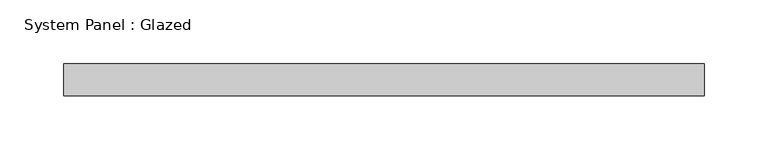
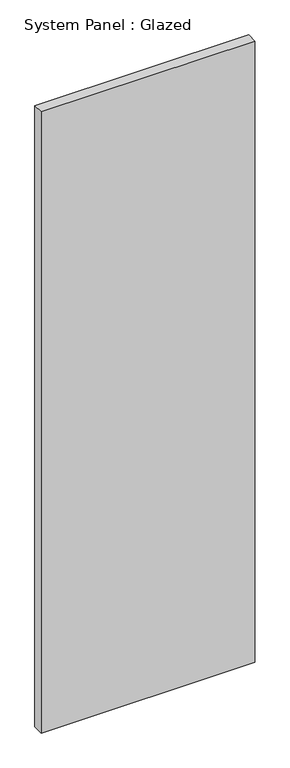
"""IFC4 building model written with IfcOpenShell, lengths in millimetres: plate geometry, System Panel : Glazed."""

from ifc_helpers import new_model, si_unit, origin, origin_with_axes, place, context, project, spatial, polyline, outline, extrude, source, transform, mapped, element, save


def system_panel_glazed_66bb8edf(model_context):
    return source(origin(), model_context, "Body", "SweptSolid", [
        extrude(outline(polyline([(251.8833333, 19.05), (-251.8833333, 19.05), (-251.8833333, 44.45), (251.8833333, 44.45), (251.8833333, 19.05)])), origin_with_axes(), (0.0, 0.0, 1.0), 1548.2875727),
    ])


if __name__ == "__main__":
    model = new_model("IFC4")
    model_context = context("Model", 3, world=origin())
    ifc_project = project(units=[si_unit("LENGTHUNIT", "METRE", prefix="MILLI")], contexts=[model_context])
    site = spatial("IfcSite", under=ifc_project)
    building = spatial("IfcBuilding", under=site)
    placement = place(None, origin())
    system_panel_glazed_shape = system_panel_glazed_66bb8edf(model_context)
    element("IfcPlate", 1, ObjectType="System Panel : Glazed", at=placement, inside=building, context=model_context, shape_type="MappedRepresentation", body=[
        mapped(system_panel_glazed_shape, transform((0.0, 0.0, 0.0), x_axis=(1.0, 0.0, 0.0), y_axis=(0.0, 1.0, 0.0), z_axis=(0.0, 0.0, 1.0))),
    ])
    save(model, "model.ifc")

# Revit data of these elements
# Type "System Panel : Glazed"
#   Construction Type Id = "GSP4R"
#   Analytic Construction = "1/8 in Pilkington single glazing"
#   Visual Light Transmittance = 0.9
#   Solar Heat Gain Coefficient = 0.86
#   Heat Transfer Coefficient (U) = 1.18115 BTU/(h·ft²·°F)
#   Define Thermal Properties by = 1
# Element 1 (IfcPlate, "System Panel : Glazed")
#   Materials on its faces: "Glass"
# Materials
#   "Glass": class "Glass", colour RGB 0 128 192, transparency 0.75, Description = "Soda Lime Glass", Cost = 0
